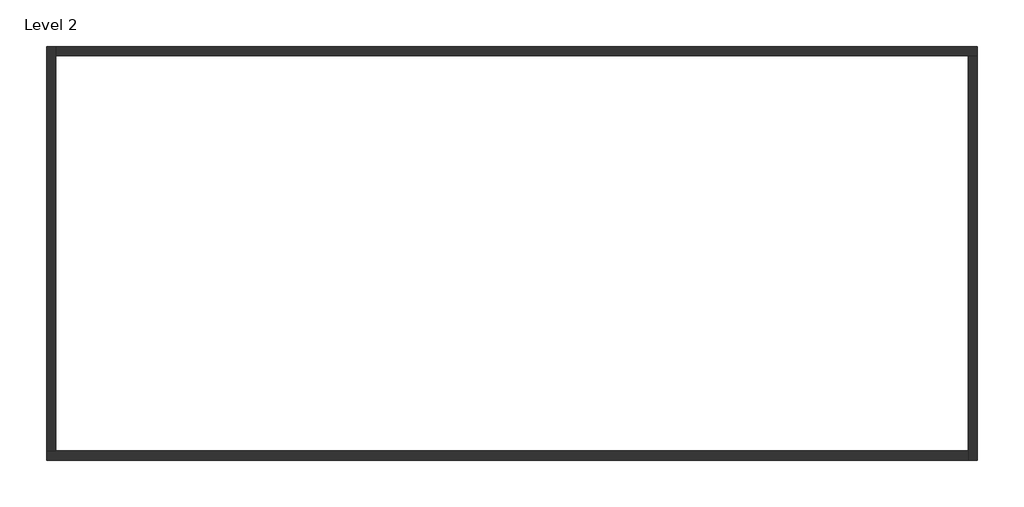
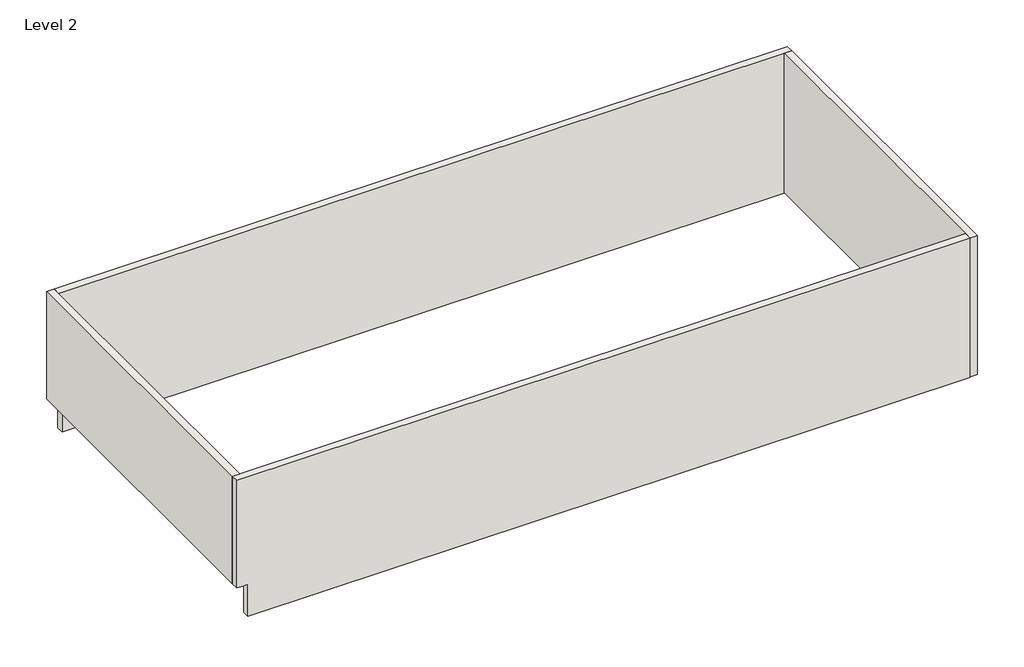
# One storey: 4 walls.
"""IFC4 building model written with IfcOpenShell, lengths in millimetres."""

from ifc_helpers import new_model, si_unit, origin, place, context, project, spatial, faceted_brep, element, save

model = new_model("IFC4")

# Units and contexts
model_context = context("Model", 3, world=origin())
ifc_project = project(units=[si_unit("LENGTHUNIT", "METRE", prefix="MILLI")], contexts=[model_context])

# Site, building, storey
site = spatial("IfcSite", under=ifc_project)
building = spatial("IfcBuilding", under=site)
storey = spatial("IfcBuildingStorey", under=building, Name="Level 2", Elevation=6096.0)

# Walls
placement = place(None, origin())
element("IfcWall", 1, ObjectType="Generic - 9\"", at=placement, inside=storey, context=model_context, shape_type="Brep", body=[
    faceted_brep([(-18712.3660557, -9535.4064876, 5182.0), (-8958.7660557, -9535.4064876, 5182.0), (-1538.7660557, -9535.4064876, 5182.0), (-1338.7660557, -9535.4064876, 5182.0), (647.2339443, -9535.4064876, 5182.0), (647.2339443, -9535.4064876, 5195.9183225), (647.2339443, -9535.4064876, 9144.0), (-19012.3660557, -9535.4064876, 9144.0), (-19012.3660557, -9535.4064876, 6096.0), (-18912.3660557, -9535.4064876, 6096.0), (-18712.3660557, -9535.4064876, 6096.0), (-18712.3660557, -9335.4064876, 5182.0), (-18712.3660557, -9335.4064876, 6096.0), (-18812.3660557, -9335.4064876, 6096.0), (-19012.3660557, -9335.4064876, 6096.0), (-19012.3660557, -9335.4064876, 9144.0), (-18812.3660557, -9335.4064876, 9144.0), (647.2339443, -9335.4064876, 9144.0), (647.2339443, -9335.4064876, 5182.0), (-1338.7660557, -9335.4064876, 5182.0), (-1538.7660557, -9335.4064876, 5182.0), (-8958.7660557, -9335.4064876, 5182.0)], [[[0, 1, 2, 3, 4, 5, 6, 7, 8, 9, 10]], [[11, 12, 13, 14, 15, 16, 17, 18, 19, 20, 21]], [[4, 3, 2, 1, 0, 11, 21, 20, 19, 18]], [[7, 6, 17, 16, 15]], [[6, 5, 4, 18, 17]], [[8, 14, 13, 12, 10, 9]], [[0, 10, 12, 11]], [[8, 7, 15, 14]]]),
])
element("IfcWall", 2, ObjectType="Generic - 9\"", at=placement, inside=storey, context=model_context, shape_type="Brep", body=[
    faceted_brep([(-19012.3660557, -701.0064876, 6096.0), (-19012.3660557, -9335.4064876, 6096.0), (-19012.3660557, -9335.4064876, 9144.0), (-19012.3660557, -701.0064876, 9144.0), (-18812.3660557, -701.0064876, 6096.0), (-18812.3660557, -701.0064876, 9144.0), (-18812.3660557, -901.0064876, 9144.0), (-18812.3660557, -9335.4064876, 9144.0), (-18812.3660557, -9335.4064876, 6096.0), (-18812.3660557, -901.0064876, 6096.0)], [[[0, 1, 2, 3]], [[4, 5, 6, 7, 8, 9]], [[1, 0, 4, 9, 8]], [[3, 2, 7, 6, 5]], [[2, 1, 8, 7]], [[0, 3, 5, 4]]]),
])
element("IfcWall", 3, ObjectType="Generic - 9\"", at=placement, inside=storey, context=model_context, shape_type="Brep", body=[
    faceted_brep([(847.2339443, -701.0064876, 5174.3674391), (-18712.3660557, -701.0064876, 5174.3674391), (-18712.3660557, -701.0064876, 6096.0), (-18812.3660557, -701.0064876, 6096.0), (-18812.3660557, -701.0064876, 9144.0), (847.2339443, -701.0064876, 9144.0), (847.2339443, -901.0064876, 5174.3674391), (847.2339443, -901.0064876, 5195.9183225), (847.2339443, -901.0064876, 9144.0), (647.2339443, -901.0064876, 9144.0), (-18812.3660557, -901.0064876, 9144.0), (-18812.3660557, -901.0064876, 6096.0), (-18712.3660557, -901.0064876, 6096.0), (-18712.3660557, -901.0064876, 5174.3674391), (-18712.3660557, -801.0064876, 6096.0)], [[[0, 1, 2, 3, 4, 5]], [[6, 7, 8, 9, 10, 11, 12, 13]], [[1, 0, 6, 13]], [[5, 4, 10, 9, 8]], [[0, 5, 8, 7, 6]], [[11, 3, 2, 14, 12]], [[2, 1, 13, 12, 14]], [[4, 3, 11, 10]]]),
])
element("IfcWall", 4, ObjectType="Generic - 9\"", at=placement, inside=storey, context=model_context, shape_type="Brep", body=[
    faceted_brep([(847.2339443, -9535.4064876, 5195.9183225), (847.2339443, -901.0064876, 5195.9183225), (847.2339443, -901.0064876, 9144.0), (847.2339443, -9535.4064876, 9144.0), (647.2339443, -9535.4064876, 5195.9183225), (647.2339443, -9535.4064876, 9144.0), (647.2339443, -9335.4064876, 9144.0), (647.2339443, -901.0064876, 9144.0), (647.2339443, -901.0064876, 5195.9183225)], [[[0, 1, 2, 3]], [[4, 5, 6, 7, 8]], [[1, 0, 4, 8]], [[3, 2, 7, 6, 5]], [[0, 3, 5, 4]], [[2, 1, 8, 7]]]),
])

save(model, "model.ifc")

# Revit data of these elements
# Type "Generic - 9\""
#   Layers, outside or top first: 200 mm no material (function 1)
# Element 1 (IfcWall, "Generic - 9\"")
#   built-in parameter 1001111 = -914 mm
#   Top Offset = 0 mm
#   Base Offset = -914 mm
#   Unconnected Height = 3962 mm
#   wall height = 3962 mm
#   Phase Created = New Construction
#   Base Constraint = Level 2
#   Materials on its faces: "Default Wall"
# Element 2 (IfcWall, "Generic - 9\"")
#   Top Offset = 0 mm
#   Base Offset = 0 mm
#   Unconnected Height = 3048 mm
#   wall height = 3048 mm
#   Phase Created = New Construction
#   Base Constraint = Level 2
#   Materials on its faces: "Default Wall"
# Element 3 (IfcWall, "Generic - 9\"")
#   built-in parameter 1001111 = -921.633 mm
#   Top Offset = 0 mm
#   Base Offset = -921.633 mm
#   Unconnected Height = 3969.633 mm
#   wall height = 3969.633 mm
#   Phase Created = New Construction
#   Base Constraint = Level 2
#   Materials on its faces: "Default Wall"
# Element 4 (IfcWall, "Generic - 9\"")
#   built-in parameter 1001111 = -900.082 mm
#   Top Offset = 0 mm
#   Base Offset = -900.082 mm
#   Unconnected Height = 3948.082 mm
#   wall height = 3948.082 mm
#   Phase Created = New Construction
#   Base Constraint = Level 2
#   Materials on its faces: "Default Wall"
# Materials
#   "Default Wall": colour RGB 80 80 80, transparency 0
